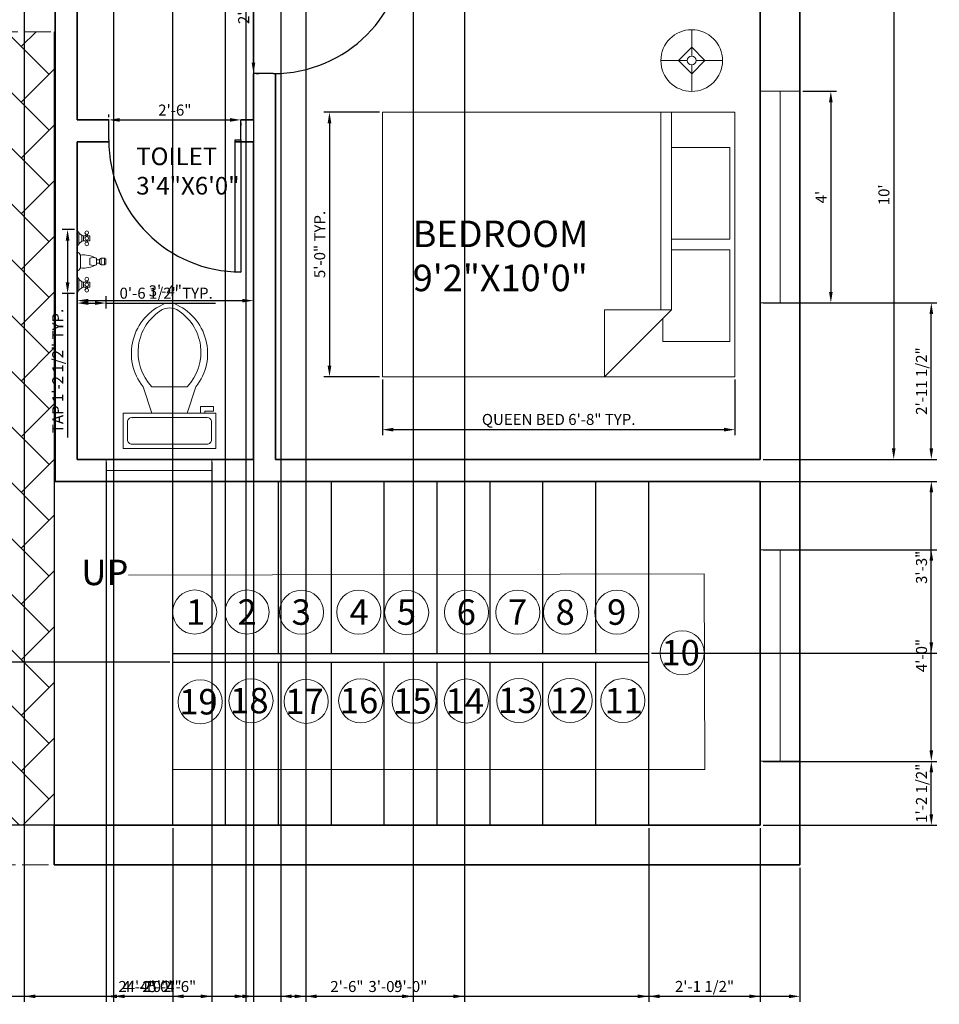
# Model space of a CAD drawing. Units: inches. Extents: x 3889 to 4254, y 3310 to 3958.
# Tile 2 of 6: x 4046 to 4254, y 3310 to 3534. Entities that reach past the tile are written whole.
import ezdxf

# ---------------------------------------------------------------- set-up
doc = ezdxf.new("R2010")
doc.units = ezdxf.units.IN
doc.linetypes.add('ACAD_ISO02W100', pattern=[15, 12, -3])
for name, color, linetype, lineweight in [('A-ANNO-SYMB', 11, 'Continuous', 18), ('A-AREA-IDEN', 11, 'Continuous', 18), ('A-FLOR-FIXT', 130, 'Continuous', 18), ('A-FLOR-OVHD', 7, 'ACAD_ISO02W100', 18), ('A-WALL', 7, 'Continuous', 35), ('DIM', 81, 'Continuous', 18), ('DOOR', 1, 'Continuous', 25), ('FLOOR', 7, 'Continuous', 25), ('FURNITURES', 130, 'Continuous', 18), ('STAIRS', 6, 'Continuous', 25), ('TEXT', 11, 'Continuous', 18), ('WINDOW', 3, 'Continuous', 18)]:
    doc.layers.add(name, color=color, linetype=linetype, lineweight=lineweight)
doc.layers.add('A-FLOR-PATT', color=215, linetype='Continuous', lineweight=13, true_color=0xa953a0)
doc.styles.get("Standard").update_dxf_attribs({"font": 'arial.ttf'})
doc.dimstyles.new('ISO-25', dxfattribs={"dimtxt": 2.5, "dimasz": 2.5, "dimexe": 1.25, "dimexo": 0.625, "dimtad": 1, "dimlunit": 3, "dimtxsty": 'Standard', "dimcen": 2.5, "dimadec": 0, "dimazin": 0, "dimtfac": 1, "dimtmove": 0, "dimatfit": 3, "dimfxl": 1, "dimarcsym": 0})

# ---------------------------------------------------------------- blocks, each defined once
blk = doc.blocks.new('*U3')
for p, q in [((-40, 0), (-40, 6)), ((0, 0), (0, 6))]:
    blk.add_line(p, q)
blk.add_lwpolyline([(0, 0), (0, -40), (-1.75, -40), (-1.75, 0)], close=True)
blk.add_arc((0, 0), 40, 180, 270)
blk = doc.blocks.new('Bed - Queen')
for p, q in [((0, -80.00003), (0, 0)), ((0, 0), (59.99999, 0)), ((59.99999, 0), (59.99999, -80.00003)), ((7.99999, -1.2), (28.79998, -1.2)), ((7.99999, -14.4), (7.99999, -1.2)), ((28.79998, -1.2), (28.79998, -14.4)), ((31.19999, -1.2), (51.99999, -1.2)), ((31.19999, -14.4), (31.19999, -1.2)), ((51.99999, -1.2), (51.99999, -16.4)), ((0, -14.4), (44.8, -14.4)), ((59.99999, -29.6), (44.8, -14.4)), ((44.8, -14.4), (44.8, -29.6)), ((44.8, -16.8), (0, -16.8)), ((51.99999, -16.4), (46.79936, -16.4)), ((44.8, -29.6), (59.99999, -29.6)), ((59.99999, -80.00003), (0, -80.00003))]:
    blk.add_line(p, q)
blk = doc.blocks.new('Lamp - Table')
for p, q in [((0, 7), (0, 1)), ((0, 3), (-3, 0)), ((3, 0), (0, 3)), ((-1, 0), (-7, 0)), ((-3, 0), (0, -3)), ((0, -3), (3, 0)), ((1, 0), (7, 0)), ((0, -1), (0, -7))]:
    blk.add_line(p, q)
for radius in [7, 1]:
    blk.add_circle((0, 0), radius)
blk = doc.blocks.new('Toilet - top')
for p, q in [((9.5, -6), (9.5, -2)), ((-10, -8.5), (-8, -8.5)), ((-10, -9.5), (-10, -8.5)), ((-8, -8.5), (-8, -8)), ((-7, -8), (-7, -9.5)), ((-4, -8), (-6, -14)), ((4, -8), (6, -14)), ((-7, -9.5), (-10, -9.5)), ((4, -14), (-4, -14))]:
    blk.add_line(p, q)
blk.add_lwpolyline([(10.5, -8), (10.5, 0), (-10.5, 0), (-10.5, -8)], close=True)
for points in [[(-9.5, -2), (-9.5, -6)], [(8.5, -1), (-8.5, -1)], [(-8.5, -7), (8.5, -7)]]:
    blk.add_lwpolyline(points)
for centre, radius, start, end in [((-8.62, -1.88), 0.884, 81.8699, 188.1301), ((8.62, -1.88), 0.884, 351.8699, 98.1301), ((-8.62, -6.12), 0.884, 171.8699, 278.1301), ((8.62, -6.12), 0.884, 261.8699, 8.1301), ((3.52, -21.58), 12.17, 141.4691, 247.9714), ((4.2, -21.82), 11.33, 136.3677, 238.9468), ((-3.52, -21.58), 12.17, 292.0284, 38.5307), ((-4.2, -21.82), 11.33, 301.053, 43.6321), ((0, -27.88), 4, 245.7318, 294.2682), ((0, -29), 4, 254.8605, 285.1395)]:
    blk.add_arc(centre, radius, start, end)
blk = doc.blocks.new('Faucet - Bathroom front')
for p, q in [((-0.5, 4.25), (0.5, 4.25)), ((0.5, 3.75), (-0.5, 3.75)), ((-0.25, 3), (-0.25, 3.5)), ((0.25, 3.5), (0.25, 3)), ((-4, 1.625), (-4.25, 1.625)), ((-3.25, 1.625), (-3, 1.625)), ((-0.5, 3), (0.5, 3)), ((0.5, 2), (-0.5, 2)), ((3.25, 1.625), (3, 1.625)), ((4, 1.625), (4.25, 1.625)), ((-5, 0), (-2.25, 0)), ((-4.5087, 0.25), (-2.7408, 0.25)), ((-4, 1.375), (-4.25, 1.375)), ((-3.1442, 0.75), (-4.0979, 0.75)), ((-3.25, 1.375), (-3, 1.375)), ((-1.5, 0), (1.5, 0)), ((-1, 0.5), (1, 0.5)), ((2.25, 0), (5, 0)), ((2.7413, 0.25), (4.5092, 0.25)), ((3.25, 1.375), (3, 1.375)), ((4.1058, 0.75), (3.1521, 0.75)), ((4, 1.375), (4.25, 1.375))]:
    blk.add_line(p, q)
for points in [[(-0.5, 3.75), (-0.5, 4.25)], [(-0.25, 4.5), (0.25, 4.5)], [(0.25, 3.5), (-0.25, 3.5)], [(0.5, 4.25), (0.5, 3.75)]]:
    blk.add_lwpolyline(points)
for points in [[(-4, 1), (-4, 2), (-3.25, 2), (-3.25, 1)], [(3.25, 1), (3.25, 2), (4, 2), (4, 1)]]:
    blk.add_lwpolyline(points, close=True)
for centre in [(-4.5, 1.5), (-3.625, 1.5), (-2.75, 1.5), (2.75, 1.5), (3.625, 1.5), (4.5, 1.5)]:
    blk.add_circle(centre, 0.2795)
for centre, radius, start, end in [((-0.2575, 4.2575), 0.2426, 88.22243, 181.7776), ((-0.2575, 3.7425), 0.2426, 178.2224, 271.7776), ((0.2575, 4.2575), 0.2426, 358.2224, 91.77757), ((0.2575, 3.7425), 0.2426, 268.2224, 1.777565), ((3, 1), 4.0311, 150.2551, 187.125), ((0.6413, 2.5), 1.246, 156.3417, 203.6583), ((-3, 1), 4.0311, 352.875, 29.74488), ((-0.6413, 2.5), 1.246, 336.3417, 23.65835), ((-5.375, 1.375), 1.4252, 285.2551, 344.7449), ((-1.875, 1.375), 1.4252, 195.2551, 254.7449), ((-0.7962, -0.2038), 0.7327, 106.1502, 163.8498), ((0.7962, -0.2038), 0.7327, 16.1502, 73.84979), ((1.875, 1.375), 1.4252, 285.2551, 344.7449), ((5.375, 1.375), 1.4252, 195.2551, 254.7449)]:
    blk.add_arc(centre, radius, start, end)
blk = doc.blocks.new('*D25')
at = {"layer": 'Defpoints', "color": 0, "transparency": 16777216}
for p in [(4065.99, 3511.11), (4095.99, 3511.11), (4095.99, 3511.11)]:
    blk.add_point(p, dxfattribs=at)
at = {"layer": 'DIM', "color": 0, "lineweight": -2, "transparency": 16777216}
for p, q in [((4065.99, 3511.73), (4065.99, 3512.36)), ((4068.49, 3511.11), (4093.49, 3511.11)), ((4095.99, 3510.48), (4095.99, 3509.86))]:
    blk.add_line(p, q, dxfattribs=at)
at = {"layer": 'DIM', "color": 0, "transparency": 16777216}
for points in [[(4068.49, 3511.52), (4068.49, 3510.69), (4065.99, 3511.11)], [(4093.49, 3511.52), (4093.49, 3510.69), (4095.99, 3511.11)]]:
    blk.add_solid(points, dxfattribs=at)
at = {"layer": 'DIM', "color": 0, "transparency": 16777216, "insert": (4080.99, 3513.01), "char_height": 2.5, "attachment_point": 5}
blk.add_mtext('2\'-6"', dxfattribs=at)
blk = doc.blocks.new('*D26')
at = {"layer": 'Defpoints', "color": 0, "transparency": 16777216}
for p in [(4098.84, 3470.11), (4058.84, 3466.61), (4098.84, 3466.61)]:
    blk.add_point(p, dxfattribs=at)
at = {"layer": 'DIM', "color": 0, "lineweight": -2, "transparency": 16777216}
for p, q in [((4058.84, 3467.23), (4058.84, 3471.36)), ((4098.84, 3467.23), (4098.84, 3471.36)), ((4061.34, 3470.11), (4096.34, 3470.11))]:
    blk.add_line(p, q, dxfattribs=at)
at = {"layer": 'DIM', "color": 0, "transparency": 16777216}
for points in [[(4061.34, 3470.52), (4061.34, 3469.69), (4058.84, 3470.11)], [(4096.34, 3470.52), (4096.34, 3469.69), (4098.84, 3470.11)]]:
    blk.add_solid(points, dxfattribs=at)
at = {"layer": 'DIM', "color": 0, "transparency": 16777216, "insert": (4078.84, 3472.01), "char_height": 2.5, "attachment_point": 5}
blk.add_mtext('3\'-4"', dxfattribs=at)
blk = doc.blocks.new('*D27')
at = {"layer": 'Defpoints', "color": 0, "transparency": 16777216}
for p in [(4098.84, 3551.61), (4098.84, 3551.61), (4098.84, 3521.61)]:
    blk.add_point(p, dxfattribs=at)
at = {"layer": 'DIM', "color": 0, "lineweight": -2, "transparency": 16777216}
for p, q in [((4099.47, 3551.61), (4100.09, 3551.61)), ((4098.84, 3524.11), (4098.84, 3549.11)), ((4099.47, 3521.61), (4100.09, 3521.61))]:
    blk.add_line(p, q, dxfattribs=at)
at = {"layer": 'DIM', "color": 0, "transparency": 16777216}
for points in [[(4098.43, 3549.11), (4099.26, 3549.11), (4098.84, 3551.61)], [(4098.43, 3524.11), (4099.26, 3524.11), (4098.84, 3521.61)]]:
    blk.add_solid(points, dxfattribs=at)
at = {"layer": 'DIM', "color": 0, "transparency": 16777216, "insert": (4096.94, 3536.61), "char_height": 2.5, "attachment_point": 5, "rotation": 90}
blk.add_mtext('2\'-6"', dxfattribs=at)
blk = doc.blocks.new('*D28')
at = {"layer": 'Defpoints', "color": 0, "transparency": 16777216}
for p in [(4222.84, 3517.61), (4222.84, 3469.61), (4229.84, 3469.61)]:
    blk.add_point(p, dxfattribs=at)
at = {"layer": 'DIM', "color": 0, "lineweight": -2, "transparency": 16777216}
for p, q in [((4223.47, 3517.61), (4231.09, 3517.61)), ((4229.84, 3515.11), (4229.84, 3472.11)), ((4223.47, 3469.61), (4231.09, 3469.61))]:
    blk.add_line(p, q, dxfattribs=at)
at = {"layer": 'DIM', "color": 0, "transparency": 16777216}
for points in [[(4229.43, 3515.11), (4230.26, 3515.11), (4229.84, 3517.61)], [(4229.43, 3472.11), (4230.26, 3472.11), (4229.84, 3469.61)]]:
    blk.add_solid(points, dxfattribs=at)
at = {"layer": 'DIM', "color": 0, "transparency": 16777216, "insert": (4227.97, 3493.61), "char_height": 2.5, "attachment_point": 5, "rotation": 90}
blk.add_mtext("4'", dxfattribs=at)
blk = doc.blocks.new('*D29')
at = {"layer": 'Defpoints', "color": 0, "transparency": 16777216}
for p in [(4213.84, 3554.11), (4213.84, 3434.11), (4244.11, 3434.11)]:
    blk.add_point(p, dxfattribs=at)
at = {"layer": 'DIM', "color": 0, "lineweight": -2, "transparency": 16777216}
for p, q in [((4214.47, 3554.11), (4245.36, 3554.11)), ((4244.11, 3551.61), (4244.11, 3436.61)), ((4214.47, 3434.11), (4245.36, 3434.11))]:
    blk.add_line(p, q, dxfattribs=at)
at = {"layer": 'DIM', "color": 0, "transparency": 16777216}
for points in [[(4243.7, 3551.61), (4244.53, 3551.61), (4244.11, 3554.11)], [(4243.7, 3436.61), (4244.53, 3436.61), (4244.11, 3434.11)]]:
    blk.add_solid(points, dxfattribs=at)
at = {"layer": 'DIM', "color": 0, "transparency": 16777216, "insert": (4242.21, 3494.11), "char_height": 2.5, "attachment_point": 5, "rotation": 90}
blk.add_mtext("10'", dxfattribs=at)
blk = doc.blocks.new('WIN-48x9')
blk.add_line((4.5, 48), (4.5, 0))
blk.add_lwpolyline([(0, 48), (9, 48), (9, 0), (0, 0)], close=True)
blk = doc.blocks.new('*D43')
at = {"layer": 'Defpoints', "color": 0, "transparency": 16777216}
for p in [(4128.09, 3452.85), (4208.09, 3452.85), (4208.09, 3440.85)]:
    blk.add_point(p, dxfattribs=at)
at = {"layer": 'DIM', "color": 0, "lineweight": -2, "transparency": 16777216}
for p, q in [((4128.09, 3452.22), (4128.09, 3439.6)), ((4208.09, 3452.22), (4208.09, 3439.6)), ((4130.59, 3440.85), (4205.59, 3440.85))]:
    blk.add_line(p, q, dxfattribs=at)
at = {"layer": 'DIM', "color": 0, "transparency": 16777216}
for points in [[(4130.59, 3441.27), (4130.59, 3440.43), (4128.09, 3440.85)], [(4205.59, 3441.27), (4205.59, 3440.43), (4208.09, 3440.85)]]:
    blk.add_solid(points, dxfattribs=at)
at = {"layer": 'DIM', "color": 0, "transparency": 16777216, "insert": (4168.09, 3442.84), "char_height": 2.5, "attachment_point": 5}
blk.add_mtext('QUEEN BED 6\'-8" TYP.', dxfattribs=at)
blk = doc.blocks.new('*D44')
at = {"layer": 'Defpoints', "color": 0, "transparency": 16777216}
for p in [(4128.09, 3512.85), (4116.09, 3452.85), (4128.09, 3452.85)]:
    blk.add_point(p, dxfattribs=at)
at = {"layer": 'DIM', "color": 0, "lineweight": -2, "transparency": 16777216}
for p, q in [((4127.46, 3512.85), (4114.84, 3512.85)), ((4116.09, 3510.35), (4116.09, 3455.35)), ((4127.46, 3452.85), (4114.84, 3452.85))]:
    blk.add_line(p, q, dxfattribs=at)
at = {"layer": 'DIM', "color": 0, "transparency": 16777216}
for points in [[(4115.67, 3510.35), (4116.51, 3510.35), (4116.09, 3512.85)], [(4115.67, 3455.35), (4116.51, 3455.35), (4116.09, 3452.85)]]:
    blk.add_solid(points, dxfattribs=at)
at = {"layer": 'DIM', "color": 0, "transparency": 16777216, "insert": (4114.19, 3482.85), "char_height": 2.5, "attachment_point": 5, "rotation": 90}
blk.add_mtext('5\'-0" TYP.', dxfattribs=at)
blk = doc.blocks.new('*D51')
at = {"layer": 'Defpoints', "color": 0, "transparency": 16777216}
for p in [(4058.84, 3486.24), (4056.67, 3471.74), (4058.84, 3471.74)]:
    blk.add_point(p, dxfattribs=at)
at = {"layer": 'DIM', "color": 0, "lineweight": -2, "transparency": 16777216}
for p, q in [((4058.22, 3486.24), (4055.42, 3486.24)), ((4056.67, 3483.74), (4056.67, 3474.24)), ((4058.22, 3471.74), (4055.42, 3471.74)), ((4056.67, 3471.74), (4056.67, 3439.1))]:
    blk.add_line(p, q, dxfattribs=at)
at = {"layer": 'DIM', "color": 0, "transparency": 16777216}
for points in [[(4056.25, 3483.74), (4057.08, 3483.74), (4056.67, 3486.24)], [(4056.25, 3474.24), (4057.08, 3474.24), (4056.67, 3471.74)]]:
    blk.add_solid(points, dxfattribs=at)
at = {"layer": 'DIM', "color": 0, "transparency": 16777216, "insert": (4054.75, 3454.17), "char_height": 2.5, "attachment_point": 5, "rotation": 90}
blk.add_mtext('TAP 1\'-2 1/2" TYP.', dxfattribs=at)
blk = doc.blocks.new('*D52')
at = {"layer": 'Defpoints', "color": 0, "transparency": 16777216}
for p in [(4058.84, 3471.74), (4065.37, 3471.74), (4065.37, 3469.56)]:
    blk.add_point(p, dxfattribs=at)
at = {"layer": 'DIM', "color": 0, "lineweight": -2, "transparency": 16777216}
for p, q in [((4058.84, 3471.11), (4058.84, 3468.31)), ((4065.37, 3471.11), (4065.37, 3468.31)), ((4061.34, 3469.56), (4062.87, 3469.56)), ((4065.37, 3469.56), (4090.19, 3469.56))]:
    blk.add_line(p, q, dxfattribs=at)
at = {"layer": 'DIM', "color": 0, "transparency": 16777216}
for points in [[(4061.34, 3469.98), (4061.34, 3469.15), (4058.84, 3469.56)], [(4062.87, 3469.98), (4062.87, 3469.15), (4065.37, 3469.56)]]:
    blk.add_solid(points, dxfattribs=at)
at = {"layer": 'DIM', "color": 0, "transparency": 16777216, "insert": (4079.03, 3471.48), "char_height": 2.5, "attachment_point": 5}
blk.add_mtext('0\'-6 1/2" TYP.', dxfattribs=at)
blk = doc.blocks.new('*D67')
at = {"layer": 'Defpoints', "color": 0, "transparency": 16777216}
for p in [(4080.52, 3351.11), (4188.52, 3351.11), (4188.52, 3312.31)]:
    blk.add_point(p, dxfattribs=at)
at = {"layer": 'DIM', "color": 0, "lineweight": -2, "transparency": 16777216}
for p, q in [((4080.52, 3350.48), (4080.52, 3311.06)), ((4188.52, 3350.48), (4188.52, 3311.06)), ((4083.02, 3312.31), (4186.02, 3312.31))]:
    blk.add_line(p, q, dxfattribs=at)
at = {"layer": 'DIM', "color": 0, "transparency": 16777216}
for points in [[(4083.02, 3312.72), (4083.02, 3311.89), (4080.52, 3312.31)], [(4186.02, 3312.72), (4186.02, 3311.89), (4188.52, 3312.31)]]:
    blk.add_solid(points, dxfattribs=at)
at = {"layer": 'DIM', "color": 0, "transparency": 16777216, "insert": (4134.52, 3314.21), "char_height": 2.5, "attachment_point": 5}
blk.add_mtext('9\'-0"', dxfattribs=at)
blk = doc.blocks.new('*D68')
at = {"layer": 'Defpoints', "color": 0, "transparency": 16777216}
for p in [(4188.52, 3351.11), (4213.84, 3351.11), (4213.84, 3312.31)]:
    blk.add_point(p, dxfattribs=at)
at = {"layer": 'DIM', "color": 0, "lineweight": -2, "transparency": 16777216}
for p, q in [((4188.52, 3350.48), (4188.52, 3311.06)), ((4213.84, 3350.48), (4213.84, 3311.06)), ((4191.02, 3312.31), (4211.34, 3312.31))]:
    blk.add_line(p, q, dxfattribs=at)
at = {"layer": 'DIM', "color": 0, "transparency": 16777216}
for points in [[(4191.02, 3312.72), (4191.02, 3311.89), (4188.52, 3312.31)], [(4211.34, 3312.72), (4211.34, 3311.89), (4213.84, 3312.31)]]:
    blk.add_solid(points, dxfattribs=at)
at = {"layer": 'DIM', "color": 0, "transparency": 16777216, "insert": (4201.18, 3314.22), "char_height": 2.5, "attachment_point": 5}
blk.add_mtext('2\'-1 1/2"', dxfattribs=at)
blk = doc.blocks.new('*D69')
at = {"layer": 'Defpoints', "color": 0, "transparency": 16777216}
for p in [(3895.04, 3388.11), (4080.52, 3388.11), (4080.52, 3351.11)]:
    blk.add_point(p, dxfattribs=at)
at = {"layer": 'DIM', "color": 0, "lineweight": -2, "transparency": 16777216}
for p, q in [((4079.89, 3388.11), (3893.79, 3388.11)), ((3895.04, 3353.61), (3895.04, 3385.61)), ((4079.89, 3351.11), (3893.79, 3351.11))]:
    blk.add_line(p, q, dxfattribs=at)
at = {"layer": 'DIM', "color": 0, "transparency": 16777216}
for points in [[(3894.63, 3385.61), (3895.46, 3385.61), (3895.04, 3388.11)], [(3894.63, 3353.61), (3895.46, 3353.61), (3895.04, 3351.11)]]:
    blk.add_solid(points, dxfattribs=at)
at = {"layer": 'DIM', "color": 0, "transparency": 16777216, "insert": (3893.14, 3369.61), "char_height": 2.5, "attachment_point": 5, "rotation": 90}
blk.add_mtext('3\'-1"', dxfattribs=at)
blk = doc.blocks.new('*D70')
at = {"layer": 'Defpoints', "color": 0, "transparency": 16777216}
for p in [(4188.52, 3429.11), (4252.64, 3429.11), (4188.52, 3390.11)]:
    blk.add_point(p, dxfattribs=at)
at = {"layer": 'DIM', "color": 0, "lineweight": -2, "transparency": 16777216}
for p, q in [((4189.14, 3429.11), (4253.89, 3429.11)), ((4252.64, 3392.61), (4252.64, 3426.61)), ((4189.14, 3390.11), (4253.89, 3390.11))]:
    blk.add_line(p, q, dxfattribs=at)
at = {"layer": 'DIM', "color": 0, "transparency": 16777216}
for points in [[(4252.23, 3426.61), (4253.06, 3426.61), (4252.64, 3429.11)], [(4252.23, 3392.61), (4253.06, 3392.61), (4252.64, 3390.11)]]:
    blk.add_solid(points, dxfattribs=at)
at = {"layer": 'DIM', "color": 0, "transparency": 16777216, "insert": (4250.74, 3409.61), "char_height": 2.5, "attachment_point": 5, "rotation": 90}
blk.add_mtext('3\'-3"', dxfattribs=at)
blk = doc.blocks.new('*D71')
at = {"layer": 'Defpoints', "color": 0, "transparency": 16777216}
for p in [(4092.52, 3951.91), (4080.52, 3351.11), (4092.52, 3351.11)]:
    blk.add_point(p, dxfattribs=at)
at = {"layer": 'DIM', "color": 0, "lineweight": -2, "transparency": 16777216}
for p, q in [((4080.52, 3351.73), (4080.52, 3953.16)), ((4083.02, 3951.91), (4090.02, 3951.91)), ((4092.52, 3351.73), (4092.52, 3953.16))]:
    blk.add_line(p, q, dxfattribs=at)
at = {"layer": 'DIM', "color": 0, "transparency": 16777216}
for points in [[(4083.02, 3952.32), (4083.02, 3951.49), (4080.52, 3951.91)], [(4090.02, 3952.32), (4090.02, 3951.49), (4092.52, 3951.91)]]:
    blk.add_solid(points, dxfattribs=at)
at = {"layer": 'DIM', "color": 0, "transparency": 16777216, "insert": (4086.52, 3953.81), "char_height": 2.5, "attachment_point": 5}
blk.add_mtext('1\'-0"', dxfattribs=at)
blk = doc.blocks.new('*D80')
at = {"layer": 'Defpoints', "color": 0, "transparency": 16777216}
for p in [(4213.84, 3469.61), (4252.64, 3469.61), (4213.84, 3434.11)]:
    blk.add_point(p, dxfattribs=at)
at = {"layer": 'DIM', "color": 0, "lineweight": -2, "transparency": 16777216}
for p, q in [((4214.47, 3469.61), (4253.89, 3469.61)), ((4252.64, 3436.61), (4252.64, 3467.11)), ((4214.47, 3434.11), (4253.89, 3434.11))]:
    blk.add_line(p, q, dxfattribs=at)
at = {"layer": 'DIM', "color": 0, "transparency": 16777216}
for points in [[(4252.23, 3467.11), (4253.06, 3467.11), (4252.64, 3469.61)], [(4252.23, 3436.61), (4253.06, 3436.61), (4252.64, 3434.11)]]:
    blk.add_solid(points, dxfattribs=at)
at = {"layer": 'DIM', "color": 0, "transparency": 16777216, "insert": (4250.73, 3451.86), "char_height": 2.5, "attachment_point": 5, "rotation": 90}
blk.add_mtext('2\'-11 1/2"', dxfattribs=at)
blk = doc.blocks.new('*D81')
at = {"layer": 'Defpoints', "color": 0, "transparency": 16777216}
for p in [(4213.84, 3365.61), (4252.64, 3365.61), (4213.84, 3351.11)]:
    blk.add_point(p, dxfattribs=at)
at = {"layer": 'DIM', "color": 0, "lineweight": -2, "transparency": 16777216}
for p, q in [((4214.47, 3365.61), (4253.89, 3365.61)), ((4252.64, 3353.61), (4252.64, 3363.11)), ((4214.47, 3351.11), (4253.89, 3351.11))]:
    blk.add_line(p, q, dxfattribs=at)
at = {"layer": 'DIM', "color": 0, "transparency": 16777216}
for points in [[(4252.23, 3363.11), (4253.06, 3363.11), (4252.64, 3365.61)], [(4252.23, 3353.61), (4253.06, 3353.61), (4252.64, 3351.11)]]:
    blk.add_solid(points, dxfattribs=at)
at = {"layer": 'DIM', "color": 0, "transparency": 16777216, "insert": (4250.73, 3358.36), "char_height": 2.5, "attachment_point": 5, "rotation": 90}
blk.add_mtext('1\'-2 1/2"', dxfattribs=at)
blk = doc.blocks.new('*D82')
at = {"layer": 'Defpoints', "color": 0, "transparency": 16777216}
for p in [(4213.84, 3413.61), (4252.64, 3413.61), (4213.84, 3365.61)]:
    blk.add_point(p, dxfattribs=at)
at = {"layer": 'DIM', "color": 0, "lineweight": -2, "transparency": 16777216}
for p, q in [((4214.47, 3413.61), (4253.89, 3413.61)), ((4252.64, 3368.11), (4252.64, 3411.11)), ((4214.47, 3365.61), (4253.89, 3365.61))]:
    blk.add_line(p, q, dxfattribs=at)
at = {"layer": 'DIM', "color": 0, "transparency": 16777216}
for points in [[(4252.23, 3411.11), (4253.06, 3411.11), (4252.64, 3413.61)], [(4252.23, 3368.11), (4253.06, 3368.11), (4252.64, 3365.61)]]:
    blk.add_solid(points, dxfattribs=at)
at = {"layer": 'DIM', "color": 0, "transparency": 16777216, "insert": (4250.74, 3389.61), "char_height": 2.5, "attachment_point": 5, "rotation": 90}
blk.add_mtext('4\'-0"', dxfattribs=at)
blk = doc.blocks.new('*D85')
at = {"layer": 'Defpoints', "color": 0, "transparency": 16777216}
for p in [(4110.69, 3860.11), (4146.69, 3860.11), (4146.69, 3312.31)]:
    blk.add_point(p, dxfattribs=at)
at = {"layer": 'DIM', "color": 0, "lineweight": -2, "transparency": 16777216}
for p, q in [((4110.69, 3859.48), (4110.69, 3311.06)), ((4146.69, 3859.48), (4146.69, 3311.06)), ((4113.19, 3312.31), (4144.19, 3312.31))]:
    blk.add_line(p, q, dxfattribs=at)
at = {"layer": 'DIM', "color": 0, "transparency": 16777216}
for points in [[(4113.19, 3312.72), (4113.19, 3311.89), (4110.69, 3312.31)], [(4144.19, 3312.72), (4144.19, 3311.89), (4146.69, 3312.31)]]:
    blk.add_solid(points, dxfattribs=at)
at = {"layer": 'DIM', "color": 0, "transparency": 16777216, "insert": (4128.69, 3314.21), "char_height": 2.5, "attachment_point": 5}
blk.add_mtext('3\'-0"', dxfattribs=at)
blk = doc.blocks.new('*D86')
at = {"layer": 'Defpoints', "color": 0, "transparency": 16777216}
for p in [(4046.84, 3865.11), (4110.69, 3865.11), (4110.69, 3312.31)]:
    blk.add_point(p, dxfattribs=at)
at = {"layer": 'DIM', "color": 0, "lineweight": -2, "transparency": 16777216}
for p, q in [((4046.84, 3864.48), (4046.84, 3311.06)), ((4110.69, 3864.48), (4110.69, 3311.06)), ((4049.34, 3312.31), (4108.19, 3312.31))]:
    blk.add_line(p, q, dxfattribs=at)
at = {"layer": 'DIM', "color": 0, "transparency": 16777216}
for points in [[(4049.34, 3312.72), (4049.34, 3311.89), (4046.84, 3312.31)], [(4108.19, 3312.72), (4108.19, 3311.89), (4110.69, 3312.31)]]:
    blk.add_solid(points, dxfattribs=at)
at = {"layer": 'DIM', "color": 0, "transparency": 16777216, "insert": (4078.77, 3314.2), "char_height": 2.5, "attachment_point": 5}
blk.add_mtext('5\'-4"', dxfattribs=at)
blk = doc.blocks.new('*D89')
at = {"layer": 'Defpoints', "color": 0, "transparency": 16777216}
for p in [(4067.08, 3735.11), (4097.08, 3735.11), (4097.08, 3312.31)]:
    blk.add_point(p, dxfattribs=at)
at = {"layer": 'DIM', "color": 0, "lineweight": -2, "transparency": 16777216}
for p, q in [((4067.08, 3734.48), (4067.08, 3311.06)), ((4097.08, 3734.48), (4097.08, 3311.06)), ((4069.58, 3312.31), (4094.58, 3312.31))]:
    blk.add_line(p, q, dxfattribs=at)
at = {"layer": 'DIM', "color": 0, "transparency": 16777216}
for points in [[(4069.58, 3312.72), (4069.58, 3311.89), (4067.08, 3312.31)], [(4094.58, 3312.72), (4094.58, 3311.89), (4097.08, 3312.31)]]:
    blk.add_solid(points, dxfattribs=at)
at = {"layer": 'DIM', "color": 0, "transparency": 16777216, "insert": (4082.08, 3314.21), "char_height": 2.5, "attachment_point": 5}
blk.add_mtext('2\'-6"', dxfattribs=at)
blk = doc.blocks.new('*D90')
at = {"layer": 'Defpoints', "color": 0, "transparency": 16777216}
for p in [(4105.04, 3735.11), (4135.04, 3735.11), (4135.04, 3312.31)]:
    blk.add_point(p, dxfattribs=at)
at = {"layer": 'DIM', "color": 0, "lineweight": -2, "transparency": 16777216}
for p, q in [((4105.04, 3734.48), (4105.04, 3311.06)), ((4135.04, 3734.48), (4135.04, 3311.06)), ((4107.54, 3312.31), (4132.54, 3312.31))]:
    blk.add_line(p, q, dxfattribs=at)
at = {"layer": 'DIM', "color": 0, "transparency": 16777216}
for points in [[(4107.54, 3312.72), (4107.54, 3311.89), (4105.04, 3312.31)], [(4132.54, 3312.72), (4132.54, 3311.89), (4135.04, 3312.31)]]:
    blk.add_solid(points, dxfattribs=at)
at = {"layer": 'DIM', "color": 0, "transparency": 16777216, "insert": (4120.04, 3314.21), "char_height": 2.5, "attachment_point": 5}
blk.add_mtext('2\'-6"', dxfattribs=at)
blk = doc.blocks.new('*D94')
at = {"layer": 'Defpoints', "color": 0, "transparency": 16777216}
for p in [(4065.39, 3434.11), (4089.39, 3434.11), (4089.39, 3312.31)]:
    blk.add_point(p, dxfattribs=at)
at = {"layer": 'DIM', "color": 0, "lineweight": -2, "transparency": 16777216}
for p, q in [((4065.39, 3433.48), (4065.39, 3311.06)), ((4089.39, 3433.48), (4089.39, 3311.06)), ((4067.89, 3312.31), (4086.89, 3312.31))]:
    blk.add_line(p, q, dxfattribs=at)
at = {"layer": 'DIM', "color": 0, "transparency": 16777216}
for points in [[(4067.89, 3312.72), (4067.89, 3311.89), (4065.39, 3312.31)], [(4086.89, 3312.72), (4086.89, 3311.89), (4089.39, 3312.31)]]:
    blk.add_solid(points, dxfattribs=at)
at = {"layer": 'DIM', "color": 0, "transparency": 16777216, "insert": (4077.39, 3314.21), "char_height": 2.5, "attachment_point": 5}
blk.add_mtext('2\'-0"', dxfattribs=at)
blk = doc.blocks.new('*D95')
at = {"layer": 'Defpoints', "color": 0, "transparency": 16777216}
for p in [(4046.84, 3865.11), (4098.84, 3860.11), (4098.84, 3312.31)]:
    blk.add_point(p, dxfattribs=at)
at = {"layer": 'DIM', "color": 0, "lineweight": -2, "transparency": 16777216}
for p, q in [((4046.84, 3864.48), (4046.84, 3311.06)), ((4098.84, 3859.48), (4098.84, 3311.06)), ((4049.34, 3312.31), (4096.34, 3312.31))]:
    blk.add_line(p, q, dxfattribs=at)
at = {"layer": 'DIM', "color": 0, "transparency": 16777216}
for points in [[(4049.34, 3312.72), (4049.34, 3311.89), (4046.84, 3312.31)], [(4096.34, 3312.72), (4096.34, 3311.89), (4098.84, 3312.31)]]:
    blk.add_solid(points, dxfattribs=at)
at = {"layer": 'DIM', "color": 0, "transparency": 16777216, "insert": (4072.84, 3314.18), "char_height": 2.5, "attachment_point": 5}
blk.add_mtext('4\'-4"', dxfattribs=at)
blk = doc.blocks.new('*D96')
at = {"layer": 'Defpoints', "color": 0, "transparency": 16777216}
for p in [(3924.84, 3342.11), (4222.84, 3342.11), (4222.84, 3312.31)]:
    blk.add_point(p, dxfattribs=at)
at = {"layer": 'DIM', "color": 0, "lineweight": -2, "transparency": 16777216}
for p, q in [((3924.84, 3341.48), (3924.84, 3311.06)), ((4222.84, 3341.48), (4222.84, 3311.06)), ((3927.34, 3312.31), (4220.34, 3312.31))]:
    blk.add_line(p, q, dxfattribs=at)
at = {"layer": 'DIM', "color": 0, "transparency": 16777216}
for points in [[(3927.34, 3312.72), (3927.34, 3311.89), (3924.84, 3312.31)], [(4220.34, 3312.72), (4220.34, 3311.89), (4222.84, 3312.31)]]:
    blk.add_solid(points, dxfattribs=at)
at = {"layer": 'DIM', "color": 0, "transparency": 16777216, "insert": (4073.84, 3314.21), "char_height": 2.5, "attachment_point": 5}
blk.add_mtext('24\'-10"', dxfattribs=at)

msp = doc.modelspace()

# ---------------------------------------------------------------- hatches: boundary and pattern name
at = {"layer": 'A-FLOR-PATT', "transparency": 33554477}
h = msp.add_hatch(dxfattribs=at)
h.set_pattern_fill('AR-HBONE', color=256, scale=0.088)
h.paths.add_polyline_path([(4053.652, 3531.107), (3933.843, 3531.107), (3933.843, 3351.107), (4053.652, 3351.107)])
edge = h.paths.add_edge_path(flags=16)
edge.add_ellipse((3558.368, 3480.977), major_axis=(-429.246, 0), ratio=0.8423039, start_angle=177.80146, end_angle=182.86371, ccw=False)
edge.add_ellipse((3971.102, 3414.23), major_axis=(61.824, 0), ratio=0.8423039, start_angle=72.28005, end_angle=85.91759)
edge.add_line((3974.812, 3466.211), (3959.972, 3466.211))
edge.add_ellipse((3963.682, 3414.23), major_axis=(-61.824, 0), ratio=0.8423039, start_angle=-85.91759, end_angle=-72.28005)
edge.add_ellipse((4376.415, 3480.977), major_axis=(429.246, 0), ratio=0.8423039, start_angle=177.13629, end_angle=182.19854, ccw=False)
edge.add_ellipse((3986.346, 3328.306), major_axis=(210.242, 0), ratio=0.8423039, start_angle=100.20954, end_angle=102.44463, ccw=False)
edge.add_ellipse((3931.309, 3647.605), major_axis=(-172.82, 0), ratio=0.8423039, start_angle=99.25657, end_angle=102.55493)
edge.add_line((3963.172, 3504.534), (3967.392, 3506.867))
edge.add_line((3967.392, 3506.867), (3971.612, 3504.534))
edge.add_ellipse((4003.474, 3647.605), major_axis=(172.82, 0), ratio=0.8423039, start_angle=257.44507, end_angle=260.74343)
edge.add_ellipse((3948.437, 3328.306), major_axis=(-210.242, 0), ratio=0.8423039, start_angle=257.55537, end_angle=259.79046, ccw=False)
edge = h.paths.add_edge_path(flags=0)
edge.add_line((3979.215, 3481.904), (3979.215, 3471.705))
edge.add_ellipse((3976.577, 3471.807), major_axis=(0.246, 4.366), ratio=0.6038336, start_angle=106.34259, end_angle=270.99799, ccw=False)
edge.add_line((3973.938, 3471.192), (3973.938, 3486.281))
edge.add_ellipse((3935.258, 3486.281), major_axis=(38.68, 0), ratio=0.8423039, start_angle=0, end_angle=29.43857)
edge.add_ellipse((3999.525, 3486.281), major_axis=(-38.68, 0), ratio=0.8423039, start_angle=-29.43857, end_angle=0)
edge.add_line((3960.846, 3486.281), (3960.846, 3471.192))
edge.add_ellipse((3958.207, 3471.807), major_axis=(-0.246, 4.366), ratio=0.6038336, start_angle=89.00201, end_angle=253.65741, ccw=False)
edge.add_line((3955.568, 3471.705), (3955.568, 3481.904))
edge.add_line((3955.568, 3481.904), (3959.527, 3484.662))
edge.add_line((3959.527, 3484.662), (3960.846, 3484.662))
edge.add_line((3960.846, 3484.662), (3960.846, 3486.281))
edge.add_ellipse((3999.525, 3486.281), major_axis=(-38.68, 0), ratio=0.8423039, start_angle=-29.43857, end_angle=0, ccw=False)
edge.add_ellipse((3935.258, 3486.281), major_axis=(38.68, 0), ratio=0.8423039, start_angle=0, end_angle=29.43857, ccw=False)
edge.add_line((3973.938, 3486.281), (3973.938, 3484.662))
edge.add_line((3973.938, 3484.662), (3975.256, 3484.662))
edge.add_line((3975.256, 3484.662), (3979.215, 3481.904))
edge = h.paths.add_edge_path(flags=16)
edge.add_line((3989.109, 3458.558), (3987.604, 3447.281))
edge.add_ellipse((3969.319, 3403.767), major_axis=(-54.801, 0), ratio=0.8423039, start_angle=247.20809, end_angle=265.12993)
edge.add_line((3973.242, 3449.808), (3961.541, 3449.808))
edge.add_ellipse((3965.464, 3403.767), major_axis=(54.801, 0), ratio=0.8423039, start_angle=94.87007, end_angle=112.79191)
edge.add_line((3947.179, 3447.281), (3945.675, 3458.558))
edge.add_ellipse((3963.682, 3413.617), major_axis=(-56.311, 0), ratio=0.8423039, start_angle=-85.72258, end_angle=-68.16505, ccw=False)
edge.add_line((3960.141, 3460.954), (3974.642, 3460.954))
edge.add_ellipse((3971.102, 3413.617), major_axis=(56.311, 0), ratio=0.8423039, start_angle=68.16505, end_angle=85.72258, ccw=False)
edge = h.paths.add_edge_path(flags=16)
edge.add_line((3987.604, 3411.46), (3987.604, 3398.498))
edge.add_ellipse((3967.392, 3482.057), major_axis=(101.242, 0), ratio=0.8423039, start_angle=256.40187, end_angle=283.59813, ccw=False)
edge.add_line((3947.179, 3398.498), (3947.179, 3411.46))
edge.add_ellipse((3967.392, 3495.02), major_axis=(101.242, 0), ratio=0.8423039, start_angle=256.40187, end_angle=283.59813)
edge = h.paths.add_edge_path(flags=16)
edge.add_ellipse((3985.566, 3391.775), major_axis=(-2.038, 0), ratio=0.8423039, start_angle=180, end_angle=270, ccw=False)
edge.add_line((3987.604, 3391.775), (3987.604, 3378.371))
edge.add_line((3987.604, 3378.371), (3947.179, 3378.371))
edge.add_line((3947.179, 3378.371), (3947.179, 3391.775))
edge.add_ellipse((3949.218, 3391.775), major_axis=(-2.038, 0), ratio=0.8423039, start_angle=-90, end_angle=0, ccw=False)
edge.add_line((3949.218, 3393.492), (3985.566, 3393.492))

# ---------------------------------------------------------------- linework, layer by layer
at = {"layer": 'A-ANNO-SYMB'}
for p, q in [((4070.474, 3407.872), (4201.123, 3408.144)), ((4201.123, 3408.144), (4201.216, 3363.736)), ((4201.216, 3363.736), (4080.518, 3363.736))]:
    msp.add_line(p, q, dxfattribs=at)
for centre in [(4085.494, 3399.477), (4097.384, 3399.477), (4109.722, 3399.426), (4122.73, 3399.465), (4133.605, 3399.377), (4147.163, 3399.428), (4158.817, 3399.428), (4169.616, 3399.428), (4181.303, 3399.428), (4196.124, 3390.218), (4086.734, 3379.091), (4098.281, 3379.349), (4110.781, 3379.217), (4123.158, 3379.349), (4135.278, 3379.266), (4147.14, 3379.298), (4159.065, 3379.41), (4170.709, 3379.424), (4182.664, 3379.385)]:
    msp.add_circle(centre, 5, dxfattribs=at)
at = {"layer": 'A-FLOR-OVHD', "ltscale": 0.5}
for p, q in [((3986.843, 3531.107), (4053.843, 3531.107)), ((4053.652, 3351.107), (3933.843, 3351.107)), ((3933.843, 3342.107), (4053.652, 3342.107))]:
    msp.add_line(p, q, dxfattribs=at)
at = {"layer": 'A-WALL'}
for p, q in [((4222.843, 3342.107), (4222.843, 3922.107)), ((4058.843, 3511.107), (4058.843, 3615.107)), ((4053.843, 3531.107), (4053.843, 3564.193)), ((4213.843, 3434.107), (4213.843, 3554.107)), ((4053.843, 3429.107), (4053.843, 3531.107)), ((4098.843, 3511.107), (4098.843, 3521.612)), ((4103.843, 3434.107), (4103.843, 3521.616)), ((4058.843, 3511.107), (4065.989, 3511.107)), ((4095.989, 3511.107), (4098.843, 3511.107)), ((4058.843, 3506.107), (4065.993, 3506.107)), ((4058.843, 3434.107), (4058.843, 3506.107)), ((4094.677, 3506.107), (4098.843, 3506.107)), ((4098.843, 3434.107), (4098.843, 3506.107)), ((4058.843, 3434.107), (4098.843, 3434.107)), ((4103.843, 3434.107), (4213.843, 3434.107)), ((4053.843, 3429.107), (4213.843, 3429.107)), ((4213.843, 3351.107), (4213.843, 3429.107)), ((4053.652, 3351.107), (4213.843, 3351.107)), ((4053.652, 3351.107), (4053.652, 3342.107)), ((4053.652, 3342.107), (4222.843, 3342.107))]:
    msp.add_line(p, q, dxfattribs=at)
at = {"layer": 'FLOOR'}
msp.add_line((4053.652, 3531.107), (4053.652, 3351.107), dxfattribs=at)
at = {"layer": 'STAIRS'}
for p, q in [((4080.518, 3390.107), (4080.518, 3429.107)), ((4092.518, 3390.107), (4092.518, 3429.107)), ((4104.518, 3390.107), (4104.518, 3429.107)), ((4116.518, 3390.107), (4116.518, 3429.107)), ((4128.518, 3390.107), (4128.518, 3429.107)), ((4140.518, 3390.107), (4140.518, 3429.107)), ((4152.518, 3390.107), (4152.518, 3429.107)), ((4164.518, 3390.107), (4164.518, 3429.107)), ((4176.518, 3390.107), (4176.518, 3429.107)), ((4188.518, 3351.107), (4188.518, 3429.107)), ((4080.518, 3390.107), (4188.518, 3390.107)), ((4080.518, 3351.107), (4080.518, 3388.107)), ((4080.518, 3388.107), (4188.518, 3388.107)), ((4092.518, 3351.107), (4092.518, 3388.107)), ((4104.518, 3351.107), (4104.518, 3388.107)), ((4116.518, 3351.107), (4116.518, 3388.107)), ((4128.518, 3351.107), (4128.518, 3388.107)), ((4140.518, 3351.107), (4140.518, 3388.107)), ((4152.518, 3351.107), (4152.518, 3388.107)), ((4164.518, 3351.107), (4164.518, 3388.107)), ((4176.518, 3351.107), (4176.518, 3388.107))]:
    msp.add_line(p, q, dxfattribs=at)
at = {"layer": 'WINDOW'}
msp.add_line((4065.394, 3431.607), (4089.394, 3431.607), dxfattribs=at)
msp.add_lwpolyline([(4065.394, 3434.107), (4065.394, 3429.107), (4089.394, 3429.107), (4089.394, 3434.107)], close=True, dxfattribs=at)

# ---------------------------------------------------------------- block references
at = {"layer": 'A-FLOR-FIXT', "xscale": 1.450441564443806, "yscale": 1.450441564443806, "zscale": 1.450441564443806, "rotation": 270}
msp.add_blockref('Faucet - Bathroom front', (4058.843, 3478.99), dxfattribs=at)
at = {"layer": 'A-FLOR-FIXT', "rotation": 180}
msp.add_blockref('Toilet - top', (4079.789, 3436.57), dxfattribs=at)
at = {"layer": 'DOOR', "xscale": 0.75, "yscale": 0.75, "zscale": 0.75, "rotation": 90}
msp.add_blockref('*U3', (4103.343, 3551.612), dxfattribs=at)
at = {"layer": 'DOOR', "xscale": 0.75, "yscale": 0.75, "zscale": 0.75}
msp.add_blockref('*U3', (4095.989, 3506.607), dxfattribs=at)
at = {"layer": 'FURNITURES'}
msp.add_blockref('Lamp - Table', (4198.273, 3524.575), dxfattribs=at)
at = {"layer": 'FURNITURES', "rotation": 270}
msp.add_blockref('Bed - Queen', (4208.089, 3512.849), dxfattribs=at)
at = {"layer": 'WINDOW'}
for p in [(4213.843, 3469.614), (4213.843, 3365.615)]:
    msp.add_blockref('WIN-48x9', p, dxfattribs=at)

# ---------------------------------------------------------------- texts
at = {"layer": 'A-AREA-IDEN', "attachment_point": 1}
for s, insert, char_height in [('TOILET\\P3\'4"X6\'0"', (4072.24, 3504.847), 4), ('BEDROOM\\P9\'2"X10\'0"', (4134.984, 3488.261), 6)]:
    msp.add_mtext_dynamic_manual_height_columns(s, width=76.4548, gutter_width=12.5, heights=[0], dxfattribs=dict(at, insert=insert, char_height=char_height))
at = {"layer": 'TEXT'}
for s, height, p in [('UP', 5.7707, (4059.783, 3405.581)), ('1', 5.771, (4083.553, 3396.58)), ('2', 5.771, (4095.236, 3396.58)), ('3', 5.771, (4107.494, 3396.58)), ('4', 5.771, (4120.632, 3396.58)), ('5', 5.771, (4131.357, 3396.58)), ('6', 5.771, (4144.955, 3396.58)), ('7', 5.771, (4156.567, 3396.58)), ('8', 5.771, (4167.388, 3396.58)), ('9', 5.771, (4179.071, 3396.58)), ('10', 5.7707, (4191.394, 3387.37)), ('19', 5.7707, (4081.989, 3376.243)), ('18', 5.7707, (4093.535, 3376.501)), ('17', 5.7707, (4106.042, 3376.32)), ('16', 5.7707, (4118.42, 3376.501)), ('15', 5.7707, (4130.517, 3376.418)), ('14', 5.7707, (4142.412, 3376.401)), ('13', 5.7707, (4154.326, 3376.564)), ('12', 5.7707, (4165.999, 3376.527)), ('11', 5.7707, (4178.482, 3376.488))]:
    msp.add_text(s, height=height, dxfattribs=at).set_placement(p)

# ---------------------------------------------------------------- dimensions: what is measured, and where the dimension line sits
at = {"layer": 'DIM'}
for base, p1, p2, override, picture, middle in [((4092.518, 3951.907), (4080.518, 3351.107), (4092.518, 3351.107), {"dimdec": 1, "dimlfac": 1, "dimrnd": 0, "dimzin": 1, "dimdsep": 46, "dimlunit": 4, "dimfrac": 2}, '*D71', (4086.518, 3953.808)), ((4110.69, 3312.307), (4046.843, 3865.107), (4110.69, 3865.107), {"dimdec": 1, "dimlfac": 1, "dimrnd": 0, "dimzin": 1, "dimdsep": 46, "dimlunit": 4, "dimfrac": 2}, '*D86', (4078.766, 3314.203)), ((4098.843, 3312.307), (4046.843, 3865.107), (4098.843, 3860.107), {"dimdec": 1, "dimlfac": 1, "dimrnd": 0, "dimzin": 1, "dimdsep": 46, "dimlunit": 4, "dimfrac": 2}, '*D95', (4072.843, 3314.182)), ((4146.69, 3312.307), (4110.69, 3860.107), (4146.69, 3860.107), {"dimdec": 1, "dimlfac": 1, "dimrnd": 0, "dimzin": 1, "dimdsep": 46, "dimlunit": 4, "dimfrac": 2}, '*D85', (4128.69, 3314.209)), ((4097.08, 3312.307), (4067.08, 3735.107), (4097.08, 3735.107), {"dimdec": 1, "dimlfac": 1, "dimrnd": 0, "dimzin": 1, "dimdsep": 46, "dimlunit": 4, "dimfrac": 2}, '*D89', (4082.08, 3314.208)), ((4135.044, 3312.307), (4105.044, 3735.107), (4135.044, 3735.107), {"dimdec": 1, "dimlfac": 1, "dimrnd": 0, "dimzin": 1, "dimdsep": 46, "dimlunit": 4, "dimfrac": 2}, '*D90', (4120.044, 3314.208)), ((4095.989, 3511.107), (4065.989, 3511.107), (4095.989, 3511.107), {"dimclrd": 0, "dimclre": 0, "dimclrt": 0}, '*D25', (4080.989, 3513.008)), ((4098.843, 3470.107), (4058.843, 3466.609), (4098.843, 3466.609), {"dimclrd": 0, "dimclre": 0, "dimclrt": 0}, '*D26', (4078.843, 3472.009)), ((4089.394, 3312.307), (4065.394, 3434.107), (4089.394, 3434.107), {"dimdec": 1, "dimlfac": 1, "dimrnd": 0, "dimzin": 1, "dimdsep": 46, "dimlunit": 4, "dimfrac": 2}, '*D94', (4077.394, 3314.208)), ((4188.518, 3312.307), (4080.518, 3351.107), (4188.518, 3351.107), {"dimdec": 1, "dimlfac": 1, "dimrnd": 0, "dimzin": 1, "dimdsep": 46, "dimlunit": 4, "dimfrac": 2}, '*D67', (4134.518, 3314.208)), ((4213.843, 3312.307), (4188.518, 3351.107), (4213.843, 3351.107), {"dimdec": 1, "dimlfac": 1, "dimrnd": 0, "dimzin": 1, "dimdsep": 46, "dimlunit": 4, "dimfrac": 2}, '*D68', (4201.18, 3314.225)), ((4222.843, 3312.307), (3924.843, 3342.107), (4222.843, 3342.107), {"dimdec": 1, "dimlfac": 1, "dimrnd": 0, "dimzin": 1, "dimdsep": 46, "dimlunit": 4, "dimfrac": 2}, '*D96', (4073.843, 3314.208))]:
    dim = msp.add_linear_dim(base=base, p1=p1, p2=p2, dimstyle='ISO-25', override=override, dxfattribs=at)
    dim.commit()
    dim.dimension.update_dxf_attribs({"geometry": picture, "text_midpoint": middle})
for base, p1, p2, override, picture, middle in [((4244.113, 3434.107), (4213.843, 3554.107), (4213.843, 3434.107), {"dimclrd": 0, "dimclre": 0, "dimclrt": 0}, '*D29', (4242.211, 3494.107)), ((4098.843, 3551.612), (4098.843, 3521.612), (4098.843, 3551.612), {"dimclrd": 0, "dimclre": 0, "dimclrt": 0}, '*D27', (4096.941, 3536.612)), ((4229.842, 3469.614), (4222.843, 3517.614), (4222.843, 3469.614), {"dimclrd": 0, "dimclre": 0, "dimclrt": 0}, '*D28', (4227.967, 3493.614)), ((4252.643, 3469.614), (4213.843, 3434.107), (4213.843, 3469.614), {"dimdec": 1, "dimlfac": 1, "dimrnd": 0, "dimzin": 1, "dimdsep": 46, "dimlunit": 4, "dimfrac": 2}, '*D80', (4250.725, 3451.86)), ((4252.643, 3429.107), (4188.518, 3390.107), (4188.518, 3429.107), {"dimdec": 1, "dimlfac": 1, "dimrnd": 0, "dimzin": 1, "dimdsep": 46, "dimlunit": 4, "dimfrac": 2}, '*D70', (4250.741, 3409.607)), ((4252.643, 3413.615), (4213.843, 3365.615), (4213.843, 3413.615), {"dimdec": 1, "dimlfac": 1, "dimrnd": 0, "dimzin": 1, "dimdsep": 46, "dimlunit": 4, "dimfrac": 2}, '*D82', (4250.741, 3389.615)), ((3895.043, 3388.107), (4080.518, 3351.107), (4080.518, 3388.107), {"dimdec": 1, "dimlfac": 1, "dimrnd": 0, "dimzin": 1, "dimdsep": 46, "dimlunit": 4, "dimfrac": 2}, '*D69', (3893.141, 3369.607)), ((4252.643, 3365.615), (4213.843, 3351.107), (4213.843, 3365.615), {"dimdec": 1, "dimlfac": 1, "dimrnd": 0, "dimzin": 1, "dimdsep": 46, "dimlunit": 4, "dimfrac": 2}, '*D81', (4250.725, 3358.361))]:
    dim = msp.add_linear_dim(base=base, p1=p1, p2=p2, angle=90, dimstyle='ISO-25', override=override, dxfattribs=at)
    dim.commit()
    dim.dimension.update_dxf_attribs({"geometry": picture, "text_midpoint": middle})
for base, p1, p2, text, picture, middle in [((4116.089, 3452.849), (4128.089, 3512.849), (4128.089, 3452.849), '<> TYP.', '*D44', (4114.188, 3482.849)), ((4056.667, 3471.738), (4058.843, 3486.242), (4058.843, 3471.738), 'TAP <> TYP.', '*D51', (4054.75, 3454.168))]:
    dim = msp.add_linear_dim(base=base, p1=p1, p2=p2, angle=270, text=text, dimstyle='ISO-25', override={"dimdec": 1, "dimlfac": 1, "dimrnd": 0, "dimzin": 1, "dimdsep": 46, "dimlunit": 4, "dimfrac": 2}, dxfattribs=at)
    dim.commit()
    dim.dimension.update_dxf_attribs({"geometry": picture, "text_midpoint": middle})
for base, p1, p2, text, picture, middle in [((4065.373, 3469.562), (4058.843, 3471.738), (4065.373, 3471.738), '<> TYP.', '*D52', (4079.03, 3471.48)), ((4208.089, 3440.849), (4128.089, 3452.849), (4208.089, 3452.849), 'QUEEN BED <> TYP.', '*D43', (4168.089, 3442.844))]:
    dim = msp.add_linear_dim(base=base, p1=p1, p2=p2, text=text, dimstyle='ISO-25', override={"dimdec": 1, "dimlfac": 1, "dimrnd": 0, "dimzin": 1, "dimdsep": 46, "dimlunit": 4, "dimfrac": 2}, dxfattribs=at)
    dim.commit()
    dim.dimension.update_dxf_attribs({"geometry": picture, "text_midpoint": middle})

doc.saveas('drawing.dxf')
